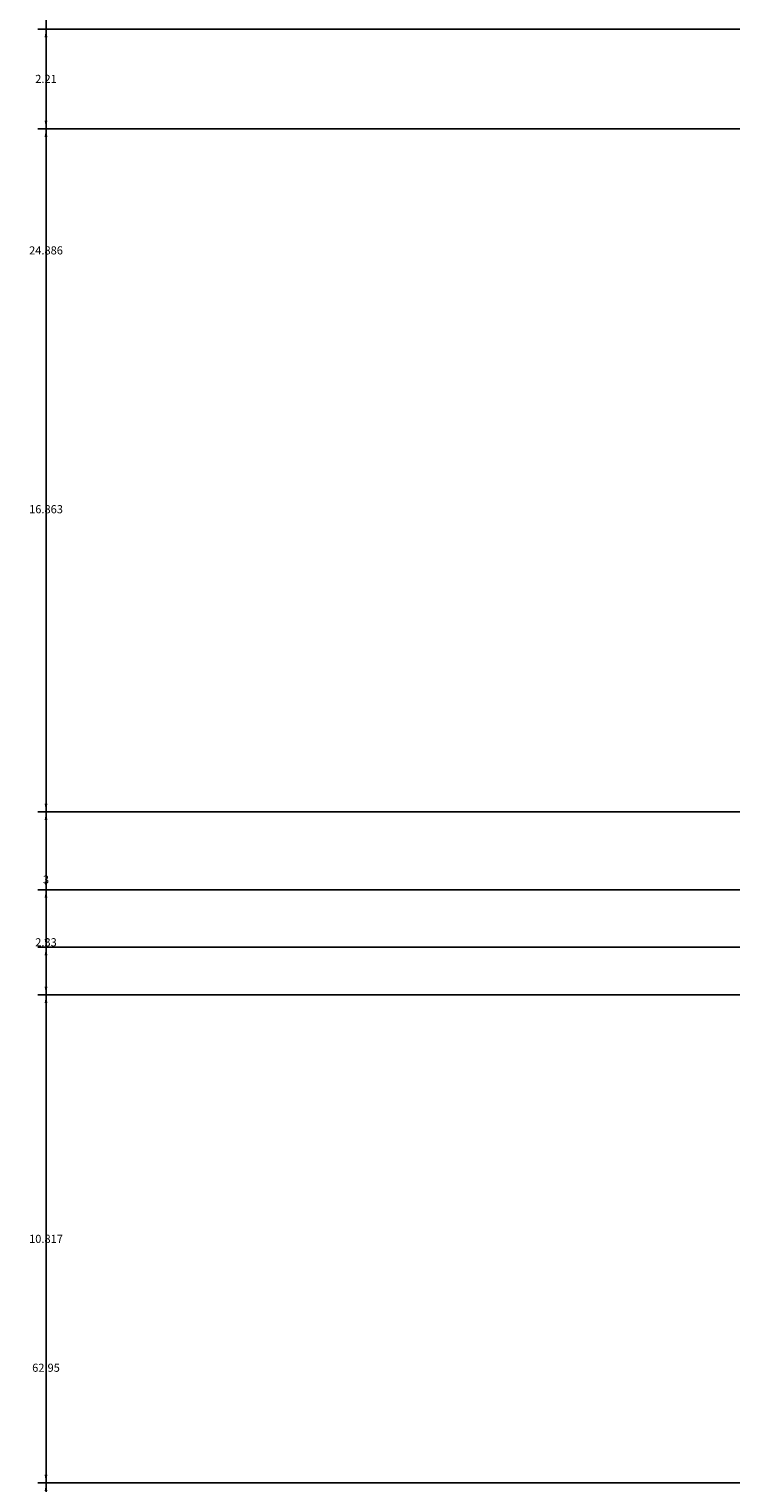
# Model space of a CAD drawing. Units: inches. Extents: x -6 to 289, y -8 to 323.
# Tile 5 of 107: x -6 to 10, y 36 to 68. Entities that reach past the tile are written whole.
import ezdxf

# ---------------------------------------------------------------- set-up
doc = ezdxf.new("R2010")
doc.units = ezdxf.units.IN
doc.header["$MEASUREMENT"] = 0
doc.layers.add('A-ANNO-DIMS', color=2, linetype='Continuous', lineweight=18)
doc.styles.get("Standard").update_dxf_attribs({"font": 'arial.ttf'})
doc.dimstyles.get("Standard").update_dxf_attribs({"dimtxt": 0.18, "dimasz": 0.18, "dimexe": 0.18, "dimexo": 0.0625, "dimgap": 0.09, "dimtad": 0, "dimtih": 1, "dimtoh": 1, "dimdec": 4, "dimzin": 0, "dimdsep": 46, "dimtxsty": 'Standard', "dimcen": 0.09, "dimadec": 0, "dimazin": 0, "dimtfac": 1, "dimtdec": 4, "dimtofl": 0, "dimtmove": 0, "dimatfit": 3, "dimfxl": 1, "dimtolj": 1, "dimtzin": 0, "dimarcsym": 0})

# ---------------------------------------------------------------- blocks, each defined once
blk = doc.blocks.new('*D17')
at = {"layer": 'A-ANNO-DIMS', "color": 0, "lineweight": -2, "transparency": 16777216}
for p, q in [((33.681, 70.243), (-5.737, 70.243)), ((-5.557, 70.063), (-5.557, 38.948)), ((-5.557, 7.469), (-5.557, 38.584)), ((11.907, 7.289), (-5.737, 7.289))]:
    blk.add_line(p, q, dxfattribs=at)
at = {"layer": 'A-ANNO-DIMS', "color": 0, "transparency": 16777216}
for points in [[(-5.587, 70.063), (-5.527, 70.063), (-5.557, 70.243)], [(-5.587, 7.469), (-5.527, 7.469), (-5.557, 7.289)]]:
    blk.add_solid(points, dxfattribs=at)
at = {"layer": 'Defpoints', "color": 0, "transparency": 16777216}
for p in [(-5.557, 70.243), (33.744, 70.243), (11.969, 7.289)]:
    blk.add_point(p, dxfattribs=at)
at = {"layer": 'A-ANNO-DIMS', "color": 0, "transparency": 16777216, "insert": (-5.557, 38.766), "char_height": 0.18, "attachment_point": 5}
blk.add_mtext('\\A1;62.95', dxfattribs=at)
blk = doc.blocks.new('*D22')
at = {"layer": 'A-ANNO-DIMS', "color": 0, "lineweight": -2, "transparency": 16777216}
for p, q in [((19.101, 307.289), (-5.737, 307.289)), ((-5.557, 307.109), (-5.557, 157.471)), ((-5.557, 7.469), (-5.557, 157.107)), ((11.907, 7.289), (-5.737, 7.289))]:
    blk.add_line(p, q, dxfattribs=at)
at = {"layer": 'A-ANNO-DIMS', "color": 0, "transparency": 16777216}
for points in [[(-5.587, 307.109), (-5.527, 307.109), (-5.557, 307.289)], [(-5.587, 7.469), (-5.527, 7.469), (-5.557, 7.289)]]:
    blk.add_solid(points, dxfattribs=at)
at = {"layer": 'Defpoints', "color": 0, "transparency": 16777216}
for p in [(19.164, 307.289), (-5.557, 7.289), (11.969, 7.289)]:
    blk.add_point(p, dxfattribs=at)
at = {"layer": 'A-ANNO-DIMS', "color": 0, "transparency": 16777216, "insert": (-5.557, 157.289), "char_height": 0.18, "attachment_point": 5}
blk.add_mtext('\\A1;300', dxfattribs=at)
blk = doc.blocks.new('*D62')
at = {"layer": 'A-ANNO-DIMS', "color": 0, "lineweight": -2, "transparency": 16777216}
for p, q in [((39.647, 36.213), (-5.737, 36.213)), ((-5.557, 36.033), (-5.557, 33.895)), ((-5.557, 31.393), (-5.557, 33.532)), ((44.647, 31.213), (-5.737, 31.213))]:
    blk.add_line(p, q, dxfattribs=at)
at = {"layer": 'A-ANNO-DIMS', "color": 0, "transparency": 16777216}
for points in [[(-5.587, 36.033), (-5.527, 36.033), (-5.557, 36.213)], [(-5.587, 31.393), (-5.527, 31.393), (-5.557, 31.213)]]:
    blk.add_solid(points, dxfattribs=at)
at = {"layer": 'Defpoints', "color": 0, "transparency": 16777216}
for p in [(-5.557, 36.213), (39.709, 36.213), (44.709, 31.213)]:
    blk.add_point(p, dxfattribs=at)
at = {"layer": 'A-ANNO-DIMS', "color": 0, "transparency": 16777216, "insert": (-5.557, 33.713), "char_height": 0.18, "attachment_point": 5}
blk.add_mtext('\\A1;5', dxfattribs=at)
blk = doc.blocks.new('*D63')
at = {"layer": 'A-ANNO-DIMS', "color": 0, "lineweight": -2, "transparency": 16777216}
for p, q in [((24.254, 47.03), (-5.737, 47.03)), ((-5.557, 46.85), (-5.557, 41.804)), ((-5.557, 36.393), (-5.557, 41.44)), ((39.647, 36.213), (-5.737, 36.213))]:
    blk.add_line(p, q, dxfattribs=at)
at = {"layer": 'A-ANNO-DIMS', "color": 0, "transparency": 16777216}
for points in [[(-5.587, 46.85), (-5.527, 46.85), (-5.557, 47.03)], [(-5.587, 36.393), (-5.527, 36.393), (-5.557, 36.213)]]:
    blk.add_solid(points, dxfattribs=at)
at = {"layer": 'Defpoints', "color": 0, "transparency": 16777216}
for p in [(-5.557, 47.03), (24.317, 47.03), (39.709, 36.213)]:
    blk.add_point(p, dxfattribs=at)
at = {"layer": 'A-ANNO-DIMS', "color": 0, "transparency": 16777216, "insert": (-5.557, 41.622), "char_height": 0.18, "attachment_point": 5}
blk.add_mtext('\\A1;10.817', dxfattribs=at)
blk = doc.blocks.new('*D64')
at = {"layer": 'A-ANNO-DIMS', "color": 0, "lineweight": -2, "transparency": 16777216}
for p, q in [((24.254, 49.36), (-5.737, 49.36)), ((-5.557, 49.18), (-5.557, 48.377)), ((-5.557, 47.21), (-5.557, 48.013)), ((24.254, 47.03), (-5.737, 47.03))]:
    blk.add_line(p, q, dxfattribs=at)
at = {"layer": 'A-ANNO-DIMS', "color": 0, "transparency": 16777216}
for points in [[(-5.587, 49.18), (-5.527, 49.18), (-5.557, 49.36)], [(-5.587, 47.21), (-5.527, 47.21), (-5.557, 47.03)]]:
    blk.add_solid(points, dxfattribs=at)
at = {"layer": 'Defpoints', "color": 0, "transparency": 16777216}
for p in [(-5.557, 49.36), (24.317, 49.36), (24.317, 47.03)]:
    blk.add_point(p, dxfattribs=at)
at = {"layer": 'A-ANNO-DIMS', "color": 0, "transparency": 16777216, "insert": (-5.557, 48.195), "char_height": 0.18, "attachment_point": 5}
blk.add_mtext('\\A1;2.33', dxfattribs=at)
blk = doc.blocks.new('*D65')
at = {"layer": 'A-ANNO-DIMS', "color": 0, "lineweight": -2, "transparency": 16777216}
for p, q in [((11.907, 66.224), (-5.737, 66.224)), ((-5.557, 66.044), (-5.557, 57.974)), ((-5.557, 49.54), (-5.557, 57.61)), ((24.254, 49.36), (-5.737, 49.36))]:
    blk.add_line(p, q, dxfattribs=at)
at = {"layer": 'A-ANNO-DIMS', "color": 0, "transparency": 16777216}
for points in [[(-5.587, 66.044), (-5.527, 66.044), (-5.557, 66.224)], [(-5.587, 49.54), (-5.527, 49.54), (-5.557, 49.36)]]:
    blk.add_solid(points, dxfattribs=at)
at = {"layer": 'Defpoints', "color": 0, "transparency": 16777216}
for p in [(-5.557, 66.224), (11.969, 66.224), (24.317, 49.36)]:
    blk.add_point(p, dxfattribs=at)
at = {"layer": 'A-ANNO-DIMS', "color": 0, "transparency": 16777216, "insert": (-5.557, 57.792), "char_height": 0.18, "attachment_point": 5}
blk.add_mtext('\\A1;16.863', dxfattribs=at)
blk = doc.blocks.new('*D66')
at = {"layer": 'A-ANNO-DIMS', "color": 0, "lineweight": -2, "transparency": 16777216}
for p, q in [((9.881, 68.432), (-5.737, 68.432)), ((-5.557, 68.252), (-5.557, 67.508)), ((-5.557, 66.404), (-5.557, 67.148)), ((11.907, 66.224), (-5.737, 66.224))]:
    blk.add_line(p, q, dxfattribs=at)
at = {"layer": 'A-ANNO-DIMS', "color": 0, "transparency": 16777216}
for points in [[(-5.587, 68.252), (-5.527, 68.252), (-5.557, 68.432)], [(-5.587, 66.404), (-5.527, 66.404), (-5.557, 66.224)]]:
    blk.add_solid(points, dxfattribs=at)
at = {"layer": 'Defpoints', "color": 0, "transparency": 16777216}
for p in [(-5.557, 68.432), (9.943, 68.432), (11.969, 66.224)]:
    blk.add_point(p, dxfattribs=at)
at = {"layer": 'A-ANNO-DIMS', "color": 0, "transparency": 16777216, "insert": (-5.557, 67.328), "char_height": 0.18, "attachment_point": 5}
blk.add_mtext('\\A1;2.21', dxfattribs=at)
blk = doc.blocks.new('*D84')
at = {"layer": 'A-ANNO-DIMS', "color": 0, "lineweight": -2, "transparency": 16777216}
for p, q in [((123.945, 48.085), (-5.737, 48.085)), ((-5.557, 47.905), (-5.557, 29.369)), ((-5.557, 10.469), (-5.557, 29.005)), ((123.945, 10.289), (-5.737, 10.289))]:
    blk.add_line(p, q, dxfattribs=at)
at = {"layer": 'A-ANNO-DIMS', "color": 0, "transparency": 16777216}
for points in [[(-5.587, 47.905), (-5.527, 47.905), (-5.557, 48.085)], [(-5.587, 10.469), (-5.527, 10.469), (-5.557, 10.289)]]:
    blk.add_solid(points, dxfattribs=at)
at = {"layer": 'Defpoints', "color": 0, "transparency": 16777216}
for p in [(-5.557, 48.085), (124.008, 48.085), (124.008, 10.289)]:
    blk.add_point(p, dxfattribs=at)
at = {"layer": 'A-ANNO-DIMS', "color": 0, "transparency": 16777216, "insert": (-5.557, 29.187), "char_height": 0.18, "attachment_point": 5}
blk.add_mtext('\\A1;37.8', dxfattribs=at)
blk = doc.blocks.new('*D85')
at = {"layer": 'A-ANNO-DIMS', "color": 0, "lineweight": -2, "transparency": 16777216}
for p, q in [((120.945, 51.085), (-5.737, 51.085)), ((-5.557, 50.905), (-5.557, 49.767)), ((-5.557, 48.265), (-5.557, 49.403)), ((123.945, 48.085), (-5.737, 48.085))]:
    blk.add_line(p, q, dxfattribs=at)
at = {"layer": 'A-ANNO-DIMS', "color": 0, "transparency": 16777216}
for points in [[(-5.587, 50.905), (-5.527, 50.905), (-5.557, 51.085)], [(-5.587, 48.265), (-5.527, 48.265), (-5.557, 48.085)]]:
    blk.add_solid(points, dxfattribs=at)
at = {"layer": 'Defpoints', "color": 0, "transparency": 16777216}
for p in [(-5.557, 51.085), (121.008, 51.085), (124.008, 48.085)]:
    blk.add_point(p, dxfattribs=at)
at = {"layer": 'A-ANNO-DIMS', "color": 0, "transparency": 16777216, "insert": (-5.557, 49.585), "char_height": 0.18, "attachment_point": 5}
blk.add_mtext('\\A1;3', dxfattribs=at)
blk = doc.blocks.new('*D86')
at = {"layer": 'A-ANNO-DIMS', "color": 0, "lineweight": -2, "transparency": 16777216}
for p, q in [((166.233, 75.971), (-5.737, 75.971)), ((-5.557, 75.791), (-5.557, 63.71)), ((-5.557, 51.265), (-5.557, 63.346)), ((120.945, 51.085), (-5.737, 51.085))]:
    blk.add_line(p, q, dxfattribs=at)
at = {"layer": 'A-ANNO-DIMS', "color": 0, "transparency": 16777216}
for points in [[(-5.587, 75.791), (-5.527, 75.791), (-5.557, 75.971)], [(-5.587, 51.265), (-5.527, 51.265), (-5.557, 51.085)]]:
    blk.add_solid(points, dxfattribs=at)
at = {"layer": 'Defpoints', "color": 0, "transparency": 16777216}
for p in [(-5.557, 75.971), (166.296, 75.971), (121.008, 51.085)]:
    blk.add_point(p, dxfattribs=at)
at = {"layer": 'A-ANNO-DIMS', "color": 0, "transparency": 16777216, "insert": (-5.557, 63.528), "char_height": 0.18, "attachment_point": 5}
blk.add_mtext('\\A1;24.886', dxfattribs=at)

msp = doc.modelspace()

# ---------------------------------------------------------------- dimensions: what is measured, and where the dimension line sits
at = {"layer": 'A-ANNO-DIMS'}
for base, p1, p2, override, picture, middle in [((-5.557, 7.2888), (19.1638, 307.2888), (11.9692, 7.2888), {"dimdec": 0, "dimlfac": 1, "dimrnd": 0, "dimzin": 0, "dimdsep": 46, "dimlunit": 2}, '*D22', (-5.557, 157.2888)), ((-5.557, 75.97064), (121.00798, 51.08513), (166.29599, 75.97064), {"dimdec": 3, "dimlfac": 1, "dimrnd": 0, "dimzin": 0, "dimdsep": 46, "dimlunit": 2}, '*D86', (-5.557, 63.52788)), ((-5.557, 70.2425), (11.9692, 7.2888), (33.7437, 70.2425), {"dimdec": 2, "dimlfac": 1, "dimrnd": 0, "dimzin": 0, "dimdsep": 46, "dimlunit": 2}, '*D17', (-5.557, 38.7657)), ((-5.557, 68.4322), (11.9692, 66.2238), (9.943, 68.4322), {"dimdec": 2, "dimlfac": 1, "dimrnd": 0, "dimzin": 0, "dimdsep": 46, "dimlunit": 2}, '*D66', (-5.557, 67.328)), ((-5.557, 66.2238), (24.317, 49.3604), (11.9692, 66.2238), {"dimdec": 3, "dimlfac": 1, "dimrnd": 0, "dimzin": 0, "dimdsep": 46, "dimlunit": 2}, '*D65', (-5.557, 57.7921)), ((-5.557, 51.0851), (124.008, 48.0851), (121.008, 51.0851), {"dimdec": 0, "dimlfac": 1, "dimrnd": 0, "dimzin": 0, "dimdsep": 46, "dimlunit": 2}, '*D85', (-5.557, 49.5851)), ((-5.557, 49.3604), (24.317, 47.0304), (24.317, 49.3604), {"dimdec": 2, "dimlfac": 1, "dimrnd": 0, "dimzin": 0, "dimdsep": 46, "dimlunit": 2}, '*D64', (-5.557, 48.1954)), ((-5.557, 48.0851), (124.008, 10.2888), (124.008, 48.0851), {"dimdec": 1, "dimlfac": 1, "dimrnd": 0, "dimzin": 0, "dimdsep": 46, "dimlunit": 2}, '*D84', (-5.557, 29.187)), ((-5.557, 47.0304), (39.709, 36.2133), (24.317, 47.0304), {"dimdec": 3, "dimlfac": 1, "dimrnd": 0, "dimzin": 0, "dimdsep": 46, "dimlunit": 2}, '*D63', (-5.557, 41.6219)), ((-5.557, 36.2133), (44.709, 31.2133), (39.709, 36.2133), {"dimdec": 0, "dimlfac": 1, "dimrnd": 0, "dimzin": 0, "dimdsep": 46, "dimlunit": 2}, '*D62', (-5.557, 33.7133))]:
    dim = msp.add_linear_dim(base=base, p1=p1, p2=p2, angle=90, dimstyle='Standard', override=override, dxfattribs=at)
    dim.commit()
    dim.dimension.update_dxf_attribs({"geometry": picture, "text_midpoint": middle})

doc.saveas('drawing.dxf')
